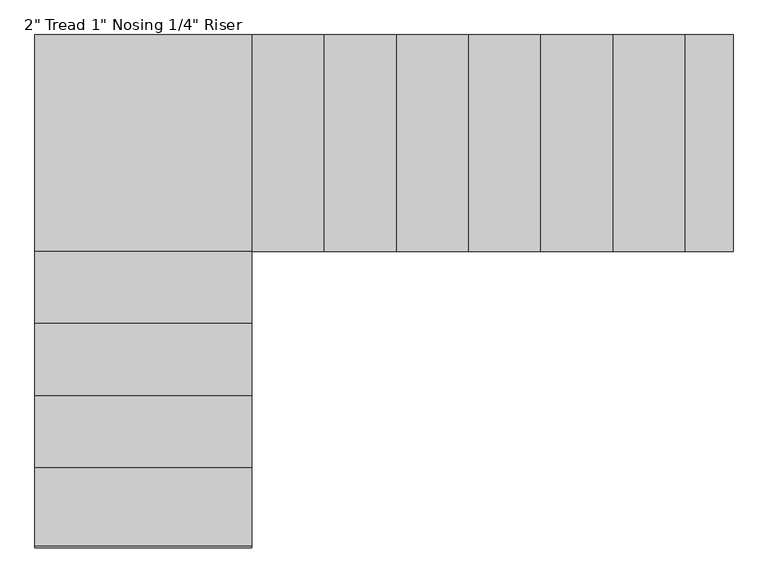
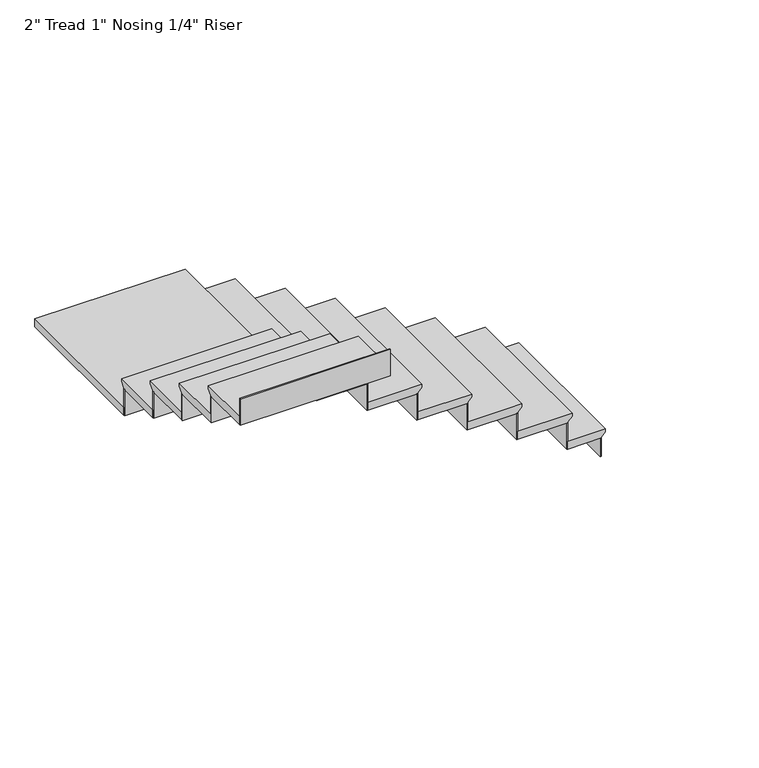
"""IFC4 building model written with IfcOpenShell, lengths in millimetres: stair flight geometry."""

from ifc_helpers import new_model, si_unit, origin, place, context, project, spatial, faceted_brep, source, transform, mapped, element, save


def stair_flight_cb1a632b(model_context):
    return source(origin(), model_context, "Body", "Brep", [
        faceted_brep([(-442.4415084, 5282.3381995, 12799.4833333), (-442.4415084, 5282.3381995, 12818.5333333), (-442.4415084, 4368.3146777, 12818.5333333), (-442.4415084, 4368.3146777, 12799.4833333), (-467.8415084, 5282.3381995, 12774.0833333), (-467.8415084, 4368.3146777, 12774.0833333), (-671.0415084, 5282.3381995, 12818.5333333), (-671.0415084, 4368.3146777, 12818.5333333), (-467.8415084, 4368.3146777, 12767.7333333), (-671.0415084, 4368.3146777, 12767.7333333), (-671.0415084, 5282.3381995, 12767.7333333), (-467.8415084, 5282.3381995, 12767.7333333)], [[[0, 1, 2, 3]], [[4, 0, 3, 5]], [[2, 1, 6, 7]], [[8, 9, 10, 11]], [[2, 7, 9, 8, 5, 3]], [[8, 11, 4, 5]], [[6, 1, 0, 4, 11, 10]], [[7, 6, 10, 9]]]),
        faceted_brep([(-467.8415084, 5282.3381995, 12767.7333333), (-467.8415084, 5282.3381995, 12649.2), (-474.1915084, 5282.3381995, 12649.2), (-474.1915084, 5282.3381995, 12767.7333333), (-467.8415084, 4368.3146777, 12767.7333333), (-474.1915084, 4368.3146777, 12767.7333333), (-474.1915084, 4368.3146777, 12649.2), (-467.8415084, 4368.3146777, 12649.2)], [[[0, 1, 2, 3]], [[4, 5, 6, 7]], [[1, 0, 4, 7]], [[2, 1, 7, 6]], [[3, 2, 6, 5]], [[0, 3, 5, 4]]]),
        faceted_brep([(-671.0415084, 5282.3381995, 12937.0666667), (-671.0415084, 5282.3381995, 12767.7333333), (-677.3915084, 5282.3381995, 12767.7333333), (-677.3915084, 5282.3381995, 12937.0666667), (-671.0415084, 4368.3146777, 12937.0666667), (-677.3915084, 4368.3146777, 12937.0666667), (-677.3915084, 4368.3146777, 12767.7333333), (-671.0415084, 4368.3146777, 12767.7333333)], [[[0, 1, 2, 3]], [[4, 5, 6, 7]], [[1, 0, 4, 7]], [[2, 1, 7, 6]], [[3, 2, 6, 5]], [[0, 3, 5, 4]]]),
        faceted_brep([(-645.6415084, 4368.3146777, 12987.8666667), (-645.6415084, 5282.3381995, 12987.8666667), (-975.8415084, 5282.3381995, 12987.8666667), (-975.8415084, 4368.3146777, 12987.8666667), (-671.0415084, 4368.3146777, 12937.0666667), (-975.8415084, 4368.3146777, 12937.0666667), (-975.8415084, 5282.3381995, 12937.0666667), (-671.0415084, 5282.3381995, 12937.0666667), (-671.0415084, 4368.3146777, 12943.4166667), (-645.6415084, 4368.3146777, 12968.8166667), (-671.0415084, 5282.3381995, 12943.4166667), (-645.6415084, 5282.3381995, 12968.8166667)], [[[0, 1, 2, 3]], [[4, 5, 6, 7]], [[0, 3, 5, 4, 8, 9]], [[4, 7, 10, 8]], [[2, 1, 11, 10, 7, 6]], [[3, 2, 6, 5]], [[11, 1, 0, 9]], [[10, 11, 9, 8]]]),
        faceted_brep([(-975.8415084, 5282.3381995, 13106.4), (-975.8415084, 5282.3381995, 12937.0666667), (-982.1915084, 5282.3381995, 12937.0666667), (-982.1915084, 5282.3381995, 13106.4), (-975.8415084, 4368.3146777, 13106.4), (-982.1915084, 4368.3146777, 13106.4), (-982.1915084, 4368.3146777, 12937.0666667), (-975.8415084, 4368.3146777, 12937.0666667)], [[[0, 1, 2, 3]], [[4, 5, 6, 7]], [[1, 0, 4, 7]], [[2, 1, 7, 6]], [[3, 2, 6, 5]], [[0, 3, 5, 4]]]),
        faceted_brep([(-950.4415084, 4368.3146777, 13157.2), (-950.4415084, 5282.3381995, 13157.2), (-1280.6415084, 5282.3381995, 13157.2), (-1280.6415084, 4368.3146777, 13157.2), (-975.8415084, 4368.3146777, 13106.4), (-1280.6415084, 4368.3146777, 13106.4), (-1280.6415084, 5282.3381995, 13106.4), (-975.8415084, 5282.3381995, 13106.4), (-975.8415084, 4368.3146777, 13112.75), (-950.4415084, 4368.3146777, 13138.15), (-975.8415084, 5282.3381995, 13112.75), (-950.4415084, 5282.3381995, 13138.15)], [[[0, 1, 2, 3]], [[4, 5, 6, 7]], [[0, 3, 5, 4, 8, 9]], [[4, 7, 10, 8]], [[2, 1, 11, 10, 7, 6]], [[3, 2, 6, 5]], [[11, 1, 0, 9]], [[10, 11, 9, 8]]]),
        faceted_brep([(-1280.6415084, 5282.3381995, 13275.7333333), (-1280.6415084, 5282.3381995, 13106.4), (-1286.9915084, 5282.3381995, 13106.4), (-1286.9915084, 5282.3381995, 13275.7333333), (-1280.6415084, 4368.3146777, 13275.7333333), (-1286.9915084, 4368.3146777, 13275.7333333), (-1286.9915084, 4368.3146777, 13106.4), (-1280.6415084, 4368.3146777, 13106.4)], [[[0, 1, 2, 3]], [[4, 5, 6, 7]], [[1, 0, 4, 7]], [[2, 1, 7, 6]], [[3, 2, 6, 5]], [[0, 3, 5, 4]]]),
        faceted_brep([(-1255.2415084, 4368.3146777, 13326.5333333), (-1255.2415084, 5282.3381995, 13326.5333333), (-1585.4415084, 5282.3381995, 13326.5333333), (-1585.4415084, 4368.3146777, 13326.5333333), (-1280.6415084, 4368.3146777, 13275.7333333), (-1585.4415084, 4368.3146777, 13275.7333333), (-1585.4415084, 5282.3381995, 13275.7333333), (-1280.6415084, 5282.3381995, 13275.7333333), (-1280.6415084, 4368.3146777, 13282.0833333), (-1255.2415084, 4368.3146777, 13307.4833333), (-1280.6415084, 5282.3381995, 13282.0833333), (-1255.2415084, 5282.3381995, 13307.4833333)], [[[0, 1, 2, 3]], [[4, 5, 6, 7]], [[0, 3, 5, 4, 8, 9]], [[4, 7, 10, 8]], [[2, 1, 11, 10, 7, 6]], [[3, 2, 6, 5]], [[11, 1, 0, 9]], [[10, 11, 9, 8]]]),
        faceted_brep([(-1585.4415084, 5282.3381995, 13445.0666667), (-1585.4415084, 5282.3381995, 13275.7333333), (-1591.7915084, 5282.3381995, 13275.7333333), (-1591.7915084, 5282.3381995, 13445.0666667), (-1585.4415084, 4368.3146777, 13445.0666667), (-1591.7915084, 4368.3146777, 13445.0666667), (-1591.7915084, 4368.3146777, 13275.7333333), (-1585.4415084, 4368.3146777, 13275.7333333)], [[[0, 1, 2, 3]], [[4, 5, 6, 7]], [[1, 0, 4, 7]], [[2, 1, 7, 6]], [[3, 2, 6, 5]], [[0, 3, 5, 4]]]),
        faceted_brep([(-1560.0415084, 4368.3146777, 13495.8666667), (-1560.0415084, 5282.3381995, 13495.8666667), (-1890.2415084, 5282.3381995, 13495.8666667), (-1890.2415084, 4368.3146777, 13495.8666667), (-1585.4415084, 4368.3146777, 13445.0666667), (-1890.2415084, 4368.3146777, 13445.0666667), (-1890.2415084, 5282.3381995, 13445.0666667), (-1585.4415084, 5282.3381995, 13445.0666667), (-1585.4415084, 4368.3146777, 13451.4166667), (-1560.0415084, 4368.3146777, 13476.8166667), (-1585.4415084, 5282.3381995, 13451.4166667), (-1560.0415084, 5282.3381995, 13476.8166667)], [[[0, 1, 2, 3]], [[4, 5, 6, 7]], [[0, 3, 5, 4, 8, 9]], [[4, 7, 10, 8]], [[2, 1, 11, 10, 7, 6]], [[3, 2, 6, 5]], [[11, 1, 0, 9]], [[10, 11, 9, 8]]]),
        faceted_brep([(-1890.2415084, 5282.3381995, 13614.4), (-1890.2415084, 5282.3381995, 13445.0666667), (-1896.5915084, 5282.3381995, 13445.0666667), (-1896.5915084, 5282.3381995, 13614.4), (-1890.2415084, 4368.3146777, 13614.4), (-1896.5915084, 4368.3146777, 13614.4), (-1896.5915084, 4368.3146777, 13445.0666667), (-1890.2415084, 4368.3146777, 13445.0666667)], [[[0, 1, 2, 3]], [[4, 5, 6, 7]], [[1, 0, 4, 7]], [[2, 1, 7, 6]], [[3, 2, 6, 5]], [[0, 3, 5, 4]]]),
        faceted_brep([(-1864.8415084, 4368.3146777, 13665.2), (-1864.8415084, 5282.3381995, 13665.2), (-2195.0415084, 5282.3381995, 13665.2), (-2195.0415084, 4368.3146777, 13665.2), (-1890.2415084, 4368.3146777, 13614.4), (-2195.0415084, 4368.3146777, 13614.4), (-2195.0415084, 5282.3381995, 13614.4), (-1890.2415084, 5282.3381995, 13614.4), (-1890.2415084, 4368.3146777, 13620.75), (-1864.8415084, 4368.3146777, 13646.15), (-1890.2415084, 5282.3381995, 13620.75), (-1864.8415084, 5282.3381995, 13646.15)], [[[0, 1, 2, 3]], [[4, 5, 6, 7]], [[0, 3, 5, 4, 8, 9]], [[4, 7, 10, 8]], [[2, 1, 11, 10, 7, 6]], [[3, 2, 6, 5]], [[11, 1, 0, 9]], [[10, 11, 9, 8]]]),
        faceted_brep([(-2195.0415084, 5282.3381995, 13783.7333333), (-2195.0415084, 5282.3381995, 13614.4), (-2201.3915084, 5282.3381995, 13614.4), (-2201.3915084, 5282.3381995, 13783.7333333), (-2195.0415084, 4368.3146777, 13783.7333333), (-2201.3915084, 4368.3146777, 13783.7333333), (-2201.3915084, 4368.3146777, 13614.4), (-2195.0415084, 4368.3146777, 13614.4)], [[[0, 1, 2, 3]], [[4, 5, 6, 7]], [[1, 0, 4, 7]], [[2, 1, 7, 6]], [[3, 2, 6, 5]], [[0, 3, 5, 4]]]),
        faceted_brep([(-2169.6415084, 4368.3146777, 13834.5333333), (-2169.6415084, 5282.3381995, 13834.5333333), (-2499.8415084, 5282.3381995, 13834.5333333), (-2499.8415084, 4368.3146777, 13834.5333333), (-2195.0415084, 4368.3146777, 13783.7333333), (-2499.8415084, 4368.3146777, 13783.7333333), (-2499.8415084, 5282.3381995, 13783.7333333), (-2195.0415084, 5282.3381995, 13783.7333333), (-2195.0415084, 4368.3146777, 13790.0833333), (-2169.6415084, 4368.3146777, 13815.4833333), (-2195.0415084, 5282.3381995, 13790.0833333), (-2169.6415084, 5282.3381995, 13815.4833333)], [[[0, 1, 2, 3]], [[4, 5, 6, 7]], [[0, 3, 5, 4, 8, 9]], [[4, 7, 10, 8]], [[2, 1, 11, 10, 7, 6]], [[3, 2, 6, 5]], [[11, 1, 0, 9]], [[10, 11, 9, 8]]]),
        faceted_brep([(-2499.8415084, 5282.3381995, 13953.0666667), (-2499.8415084, 5282.3381995, 13783.7333333), (-2506.1915084, 5282.3381995, 13783.7333333), (-2506.1915084, 5282.3381995, 13953.0666667), (-2499.8415084, 4368.3146777, 13953.0666667), (-2506.1915084, 4368.3146777, 13953.0666667), (-2506.1915084, 4368.3146777, 13783.7333333), (-2499.8415084, 4368.3146777, 13783.7333333)], [[[0, 1, 2, 3]], [[4, 5, 6, 7]], [[1, 0, 4, 7]], [[2, 1, 7, 6]], [[3, 2, 6, 5]], [[0, 3, 5, 4]]]),
        faceted_brep([(-3388.8415084, 5282.3381995, 14003.8666667), (-3388.8415084, 4342.9146777, 14003.8666667), (-2474.4415084, 4342.9146777, 14003.8666667), (-2474.4415084, 5282.3381995, 14003.8666667), (-2474.4415084, 4368.3146777, 13953.0666667), (-2474.4415084, 4342.9146777, 13953.0666667), (-3388.8415084, 4342.9146777, 13953.0666667), (-3388.8415084, 5282.3381995, 13953.0666667), (-2499.8415084, 5282.3381995, 13953.0666667), (-2499.8415084, 4368.3146777, 13953.0666667), (-2474.4415084, 4368.3146777, 13984.8166667), (-2474.4415084, 5282.3381995, 13984.8166667), (-2499.8415084, 4368.3146777, 13959.4166667), (-2499.8415084, 5282.3381995, 13959.4166667)], [[[0, 1, 2, 3]], [[4, 5, 6, 7, 8, 9]], [[3, 2, 5, 4, 10, 11]], [[4, 9, 12, 10]], [[9, 8, 13, 12]], [[0, 3, 11, 13, 8, 7]], [[1, 0, 7, 6]], [[2, 1, 6, 5]], [[13, 11, 10, 12]]]),
        faceted_brep([(-3388.8415084, 4342.9146777, 14122.4), (-3388.8415084, 4342.9146777, 13953.0666667), (-3388.8415084, 4336.5646777, 13953.0666667), (-3388.8415084, 4336.5646777, 14122.4), (-2474.4415084, 4342.9146777, 14122.4), (-2474.4415084, 4336.5646777, 14122.4), (-2474.4415084, 4336.5646777, 13953.0666667), (-2474.4415084, 4342.9146777, 13953.0666667)], [[[0, 1, 2, 3]], [[4, 5, 6, 7]], [[1, 0, 4, 7]], [[2, 1, 7, 6]], [[3, 2, 6, 5]], [[0, 3, 5, 4]]]),
        faceted_brep([(-2474.4415084, 4368.3146777, 14173.2), (-3388.8415084, 4368.3146777, 14173.2), (-3388.8415084, 4037.7382512, 14173.2), (-2474.4415084, 4037.7382512, 14173.2), (-2474.4415084, 4342.9146777, 14122.4), (-2474.4415084, 4037.7382512, 14122.4), (-3388.8415084, 4037.7382512, 14122.4), (-3388.8415084, 4342.9146777, 14122.4), (-2474.4415084, 4342.9146777, 14128.75), (-2474.4415084, 4368.3146777, 14154.15), (-3388.8415084, 4342.9146777, 14128.75), (-3388.8415084, 4368.3146777, 14154.15)], [[[0, 1, 2, 3]], [[4, 5, 6, 7]], [[0, 3, 5, 4, 8, 9]], [[4, 7, 10, 8]], [[2, 1, 11, 10, 7, 6]], [[3, 2, 6, 5]], [[11, 1, 0, 9]], [[10, 11, 9, 8]]]),
        faceted_brep([(-3388.8415084, 4037.7382512, 14291.7333333), (-3388.8415084, 4037.7382512, 14122.4), (-3388.8415084, 4031.3882512, 14122.4), (-3388.8415084, 4031.3882512, 14291.7333333), (-2474.4415084, 4037.7382512, 14291.7333333), (-2474.4415084, 4031.3882512, 14291.7333333), (-2474.4415084, 4031.3882512, 14122.4), (-2474.4415084, 4037.7382512, 14122.4)], [[[0, 1, 2, 3]], [[4, 5, 6, 7]], [[1, 0, 4, 7]], [[2, 1, 7, 6]], [[3, 2, 6, 5]], [[0, 3, 5, 4]]]),
        faceted_brep([(-2474.4415084, 4063.1382512, 14342.5333333), (-3388.8415084, 4063.1382512, 14342.5333333), (-3388.8415084, 3732.938277, 14342.5333333), (-2474.4415084, 3732.938277, 14342.5333333), (-2474.4415084, 4037.7382512, 14291.7333333), (-2474.4415084, 3732.938277, 14291.7333333), (-3388.8415084, 3732.938277, 14291.7333333), (-3388.8415084, 4037.7382512, 14291.7333333), (-2474.4415084, 4037.7382512, 14298.0833333), (-2474.4415084, 4063.1382512, 14323.4833333), (-3388.8415084, 4037.7382512, 14298.0833333), (-3388.8415084, 4063.1382512, 14323.4833333)], [[[0, 1, 2, 3]], [[4, 5, 6, 7]], [[0, 3, 5, 4, 8, 9]], [[4, 7, 10, 8]], [[2, 1, 11, 10, 7, 6]], [[3, 2, 6, 5]], [[11, 1, 0, 9]], [[10, 11, 9, 8]]]),
        faceted_brep([(-3388.8415084, 3732.938277, 14461.0666667), (-3388.8415084, 3732.938277, 14291.7333333), (-3388.8415084, 3726.588277, 14291.7333333), (-3388.8415084, 3726.588277, 14461.0666667), (-2474.4415084, 3732.938277, 14461.0666667), (-2474.4415084, 3726.588277, 14461.0666667), (-2474.4415084, 3726.588277, 14291.7333333), (-2474.4415084, 3732.938277, 14291.7333333)], [[[0, 1, 2, 3]], [[4, 5, 6, 7]], [[1, 0, 4, 7]], [[2, 1, 7, 6]], [[3, 2, 6, 5]], [[0, 3, 5, 4]]]),
        faceted_brep([(-2474.4415084, 3758.338277, 14511.8666667), (-3388.8415084, 3758.338277, 14511.8666667), (-3388.8415084, 3428.1383028, 14511.8666667), (-2474.4415084, 3428.1383028, 14511.8666667), (-2474.4415084, 3732.938277, 14461.0666667), (-2474.4415084, 3428.1383028, 14461.0666667), (-3388.8415084, 3428.1383028, 14461.0666667), (-3388.8415084, 3732.938277, 14461.0666667), (-2474.4415084, 3732.938277, 14467.4166667), (-2474.4415084, 3758.338277, 14492.8166667), (-3388.8415084, 3732.938277, 14467.4166667), (-3388.8415084, 3758.338277, 14492.8166667)], [[[0, 1, 2, 3]], [[4, 5, 6, 7]], [[0, 3, 5, 4, 8, 9]], [[4, 7, 10, 8]], [[2, 1, 11, 10, 7, 6]], [[3, 2, 6, 5]], [[11, 1, 0, 9]], [[10, 11, 9, 8]]]),
        faceted_brep([(-3388.8415084, 3428.1383028, 14630.4), (-3388.8415084, 3428.1383028, 14461.0666667), (-3388.8415084, 3421.7883028, 14461.0666667), (-3388.8415084, 3421.7883028, 14630.4), (-2474.4415084, 3428.1383028, 14630.4), (-2474.4415084, 3421.7883028, 14630.4), (-2474.4415084, 3421.7883028, 14461.0666667), (-2474.4415084, 3428.1383028, 14461.0666667)], [[[0, 1, 2, 3]], [[4, 5, 6, 7]], [[1, 0, 4, 7]], [[2, 1, 7, 6]], [[3, 2, 6, 5]], [[0, 3, 5, 4]]]),
        faceted_brep([(-3388.8415084, 3123.3383287, 14799.7333333), (-3388.8415084, 3123.3383287, 14630.4), (-3388.8415084, 3116.9883287, 14630.4), (-3388.8415084, 3116.9883287, 14799.7333333), (-2474.4415084, 3123.3383287, 14799.7333333), (-2474.4415084, 3116.9883287, 14799.7333333), (-2474.4415084, 3116.9883287, 14630.4), (-2474.4415084, 3123.3383287, 14630.4)], [[[0, 1, 2, 3]], [[4, 5, 6, 7]], [[1, 0, 4, 7]], [[2, 1, 7, 6]], [[3, 2, 6, 5]], [[0, 3, 5, 4]]]),
        faceted_brep([(-2474.4415084, 3453.5383028, 14681.2), (-3388.8415084, 3453.5383028, 14681.2), (-3388.8415084, 3123.3383287, 14681.2), (-2474.4415084, 3123.3383287, 14681.2), (-2474.4415084, 3428.1383028, 14630.4), (-2474.4415084, 3123.3383287, 14630.4), (-3388.8415084, 3123.3383287, 14630.4), (-3388.8415084, 3428.1383028, 14630.4), (-2474.4415084, 3428.1383028, 14636.75), (-2474.4415084, 3453.5383028, 14662.15), (-3388.8415084, 3428.1383028, 14636.75), (-3388.8415084, 3453.5383028, 14662.15)], [[[0, 1, 2, 3]], [[4, 5, 6, 7]], [[0, 3, 5, 4, 8, 9]], [[4, 7, 10, 8]], [[2, 1, 11, 10, 7, 6]], [[3, 2, 6, 5]], [[11, 1, 0, 9]], [[10, 11, 9, 8]]]),
    ])


if __name__ == "__main__":
    model = new_model("IFC4")
    model_context = context("Model", 3, world=origin())
    ifc_project = project(units=[si_unit("LENGTHUNIT", "METRE", prefix="MILLI")], contexts=[model_context])
    site = spatial("IfcSite", under=ifc_project)
    building = spatial("IfcBuilding", under=site)
    placement = place(None, origin())
    stair_flight_shape = stair_flight_cb1a632b(model_context)
    element("IfcStairFlight", 1, ObjectType="2\" Tread 1\" Nosing 1/4\" Riser", at=placement, inside=building, context=model_context, shape_type="MappedRepresentation", body=[
        mapped(stair_flight_shape, transform((0.0, 0.0, 0.0), x_axis=(1.0, 0.0, 0.0), y_axis=(0.0, 1.0, 0.0), z_axis=(0.0, 0.0, 1.0))),
    ])
    save(model, "model.ifc")
